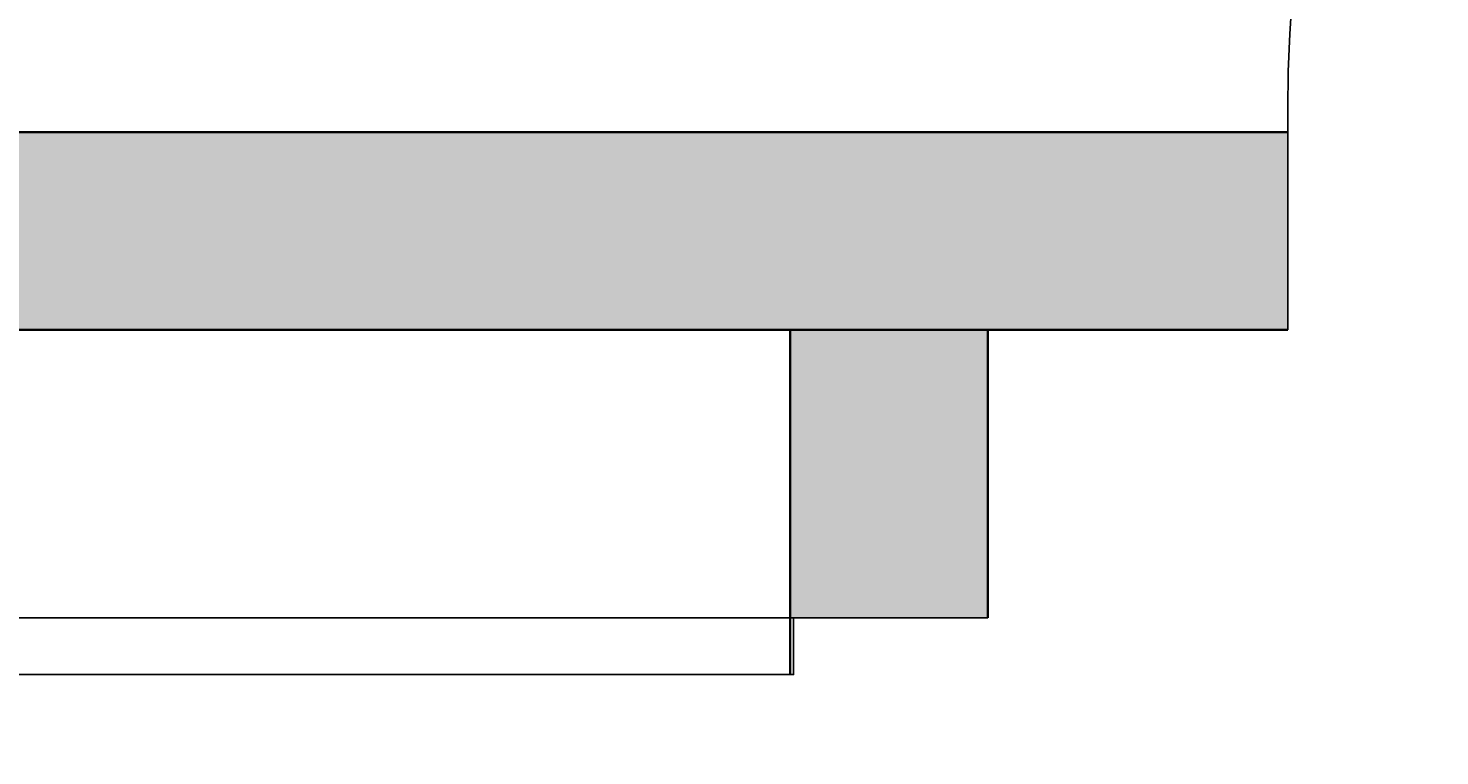
# Model space of a CAD drawing. Units: inches. Extents: x 1998 to 2588, y 1139 to 1977.
# Tile 66 of 134: x 2160 to 2192, y 1746 to 1762. Entities that reach past the tile are written whole.
import ezdxf

# ---------------------------------------------------------------- set-up
doc = ezdxf.new("R2010")
doc.units = ezdxf.units.IN
for name, color, linetype, lineweight in [('A-ANNO-DIMS', 2, 'Continuous', 18), ('A-WALL-PATT', 252, 'Continuous', 13), ('DOOR', 52, 'Continuous', 25), ('WALL', 200, 'Continuous', 35)]:
    doc.layers.add(name, color=color, linetype=linetype, lineweight=lineweight)
doc.styles.get("Standard").update_dxf_attribs({"font": 'arial.ttf'})
doc.dimstyles.get("Standard").update_dxf_attribs({"dimtxt": 0.18, "dimasz": 0.18, "dimexe": 0.18, "dimexo": 0.0625, "dimgap": 0.09, "dimtad": 0, "dimtih": 1, "dimtoh": 1, "dimdec": 4, "dimzin": 0, "dimdsep": 46, "dimtxsty": 'Standard', "dimcen": 0.09, "dimadec": 0, "dimazin": 0, "dimtfac": 1, "dimtdec": 4, "dimtofl": 0, "dimtmove": 0, "dimatfit": 3, "dimfxl": 1, "dimtolj": 1, "dimtzin": 0, "dimarcsym": 0})

# ---------------------------------------------------------------- blocks, each defined once
blk = doc.blocks.new('*U2')
for p, q in [((0, 0), (0, -6)), ((40, 0), (40, -6))]:
    blk.add_line(p, q)
blk.add_lwpolyline([(0, 0), (0, 40), (1.75, 40), (1.75, 0)], close=True)
blk.add_arc((0, 0), 40, 0, 90)
blk = doc.blocks.new('*D37')
at = {"layer": 'A-ANNO-DIMS', "color": 0, "lineweight": -2, "transparency": 16777216}
for p, q in [((2148.455, 1612.795), (2148.455, 1977.362)), ((2197.45, 1612.795), (2197.45, 1977.362)), ((2148.635, 1977.182), (2172.73, 1977.182)), ((2197.27, 1977.182), (2173.175, 1977.182))]:
    blk.add_line(p, q, dxfattribs=at)
at = {"layer": 'A-ANNO-DIMS', "color": 0, "transparency": 16777216}
for points in [[(2148.635, 1977.212), (2148.635, 1977.152), (2148.455, 1977.182)], [(2197.27, 1977.212), (2197.27, 1977.152), (2197.45, 1977.182)]]:
    blk.add_solid(points, dxfattribs=at)
at = {"layer": 'Defpoints', "color": 0, "transparency": 16777216}
for p in [(2197.45, 1977.182), (2148.455, 1612.732), (2197.45, 1612.732)]:
    blk.add_point(p, dxfattribs=at)
at = {"layer": 'A-ANNO-DIMS', "color": 0, "transparency": 16777216, "insert": (2172.952, 1977.182), "char_height": 0.18, "attachment_point": 5}
blk.add_mtext('\\A1;49', dxfattribs=at)

msp = doc.modelspace()

# ---------------------------------------------------------------- hatches: boundary and pattern name
at = {"layer": 'A-WALL-PATT'}
h = msp.add_hatch(color=256, dxfattribs=at)
h.dxf.hatch_style = 1
h.paths.add_polyline_path([(2222.9729, 1888.7324), (2099.4125, 1888.7324), (2099.4125, 1879.7324), (2222.9729, 1879.7324)])
h.paths.add_polyline_path([(2096.9729, 1868.3278), (2087.9729, 1868.3278), (2087.9729, 1775.637), (2096.9729, 1775.637)])
h.paths.add_polyline_path([(2227.4729, 1868.3278), (2222.9729, 1868.3278), (2222.9729, 1774.3318), (2227.4729, 1774.3318)])
h.paths.add_polyline_path([(2188.3019, 1759.7324), (2138.6074, 1759.7324), (2099.4125, 1759.7324), (2099.4125, 1755.2324), (2176.9729, 1755.2324), (2188.3019, 1755.2324)])
h.paths.add_polyline_path([(2087.9729, 1759.7324), (2059.4729, 1759.7324), (2059.4729, 1702.7324), (2087.9729, 1702.7324), (2087.9729, 1707.2324), (2063.9729, 1707.2324), (2063.9729, 1755.2324), (2087.9729, 1755.2324)])
h.paths.add_polyline_path([(2096.9729, 1755.2324), (2087.9729, 1755.2324), (2087.9729, 1707.2324), (2096.9729, 1707.2324)])
h.paths.add_polyline_path([(2187.0461, 1707.2324), (2105.9729, 1707.2324), (2096.9729, 1707.2324), (2087.9729, 1707.2324), (2087.9729, 1702.7324), (2105.9729, 1702.7324), (2114.9729, 1702.7324), (2187.0461, 1702.7324)])
h.paths.add_polyline_path([(2181.4729, 1719.2028), (2176.9729, 1719.2028), (2176.9729, 1707.2324), (2181.4729, 1707.2324)])
h.paths.add_polyline_path([(2216.0332, 1588.7324), (2114.9729, 1588.7324), (2105.9729, 1588.7324), (2105.9729, 1584.2324), (2216.0332, 1584.2324)])
h.paths.add_polyline_path([(2077.691, 1588.7324), (2061.4729, 1588.7324), (2061.4729, 1584.2324), (2077.691, 1584.2324)])
h.paths.add_polyline_path([(2105.9729, 1588.7324), (2098.0956, 1588.7324), (2098.0956, 1584.2324), (2105.9729, 1584.2324)])
h.paths.add_polyline_path([(2114.9729, 1596.2642), (2110.1012, 1596.2642), (2105.9729, 1596.2642), (2105.9729, 1588.7324), (2114.9729, 1588.7324)])
h.paths.add_polyline_path([(2114.9729, 1584.2324), (2105.9729, 1584.2324), (2105.9729, 1580.249), (2110.1012, 1580.249), (2114.9729, 1580.249)])
h.paths.add_polyline_path([(2114.9729, 1547.7716), (2110.1012, 1547.7716, -0.0318759), (2105.9729, 1548.035), (2105.9729, 1470.2324), (2108.3775, 1470.2324), (2108.3775, 1465.7324), (2186.2943, 1465.7324), (2186.2943, 1470.2324), (2114.9729, 1470.2324)])
h.paths.add_polyline_path([(2227.4729, 1584.2324), (2222.9729, 1584.2324), (2222.9729, 1486.137), (2227.4729, 1486.137)])
h.paths.add_polyline_path([(2295.4138, 1593.2324), (2227.4729, 1593.2324), (2227.4729, 1588.7324), (2295.4138, 1588.7324), (2295.4138, 1591.8729)])
h.paths.add_polyline_path([(2345.9729, 1627.1165), (2341.4729, 1627.1165), (2341.4729, 1593.2324), (2337.2869, 1593.2324), (2337.2869, 1591.8729), (2337.2869, 1588.7324), (2345.9729, 1588.7324)])
h.paths.add_polyline_path([(2291.9729, 1588.7324), (2287.4729, 1588.7324), (2287.4729, 1522.7324), (2291.9729, 1522.7324)])
h.paths.add_polyline_path([(2291.9729, 1522.7324), (2287.4729, 1522.7324), (2227.4729, 1522.7324), (2227.4729, 1518.2324), (2291.9729, 1518.2324)])
h.paths.add_polyline_path([(2295.7347, 1519.5919), (2295.7347, 1522.7324), (2291.9729, 1522.7324), (2291.9729, 1518.2324), (2295.7347, 1518.2324)])
h.paths.add_polyline_path([(2345.9729, 1522.7324), (2337.6078, 1522.7324), (2337.6078, 1519.5919), (2337.6078, 1518.2324), (2341.4729, 1518.2324), (2341.4729, 1488.5616), (2345.9729, 1488.5616)])
h.paths.add_polyline_path([(2345.9729, 1468.1569), (2341.4729, 1468.1569), (2341.4729, 1374.2324), (2227.4729, 1374.2324), (2227.4729, 1369.7324), (2345.9729, 1369.7324)])
h.paths.add_polyline_path([(2345.9729, 1369.7324), (2341.4729, 1369.7324), (2341.4729, 1362.2324), (2345.9729, 1362.2324)])
h.paths.add_polyline_path([(2345.9729, 1317.7324), (2345.9729, 1322.2324), (2341.4729, 1322.2324), (2341.4729, 1285.137), (2345.9729, 1285.137)], flags=17)
h.paths.add_polyline_path([(2356.2096, 1322.2324), (2345.9729, 1322.2324), (2345.9729, 1317.7324), (2356.2096, 1317.7324), (2356.2096, 1319.3088)], flags=17)
h.paths.add_polyline_path([(2393.9729, 1322.2324), (2375.6999, 1322.2324), (2375.6999, 1319.3088, -0.0202458), (2375.636, 1317.7324), (2393.9729, 1317.7324)], flags=17)
h.paths.add_polyline_path([(2398.4729, 1322.2324), (2393.9729, 1322.2324), (2393.9729, 1317.7324), (2393.9729, 1237.7324), (2345.9729, 1237.7324), (2345.9729, 1264.7324), (2341.4729, 1264.7324), (2341.4729, 1228.7324), (2393.9729, 1228.7324), (2482.7412, 1228.7324), (2482.7412, 1237.7324), (2398.4729, 1237.7324), (2398.4729, 1297.1029)])
h.paths.add_polyline_path([(2398.4729, 1362.2324), (2393.9729, 1362.2324), (2393.9729, 1357.7324), (2398.4729, 1357.7324)])
h.paths.add_polyline_path([(2345.9729, 1329.7549), (2341.4729, 1329.7549), (2341.4729, 1322.2324), (2345.9729, 1322.2324)])
h = msp.add_hatch(color=256, dxfattribs=at)
h.dxf.hatch_style = 1
h.paths.add_polyline_path([(2527.4729, 1362.2324), (2510.9729, 1362.2324), (2510.9729, 1357.7324), (2518.4729, 1357.7324), (2518.4729, 1237.7324), (2503.1458, 1237.7324), (2503.1458, 1228.7324), (2527.4729, 1228.7324)])
h.paths.add_polyline_path([(2490.5682, 1362.2324), (2398.4729, 1362.2324), (2398.4729, 1357.7324), (2490.5682, 1357.7324)])
h.paths.add_polyline_path([(2224.9729, 1264.7324), (2222.9729, 1264.7324), (2222.9729, 1232.4125), (2341.4729, 1232.4125), (2341.4729, 1234.4125), (2224.9729, 1234.4125)])
h.paths.add_polyline_path([(2334.5332, 1273.7324), (2264.7638, 1273.7324), (2264.7638, 1269.5611, -0.043659), (2264.3413, 1264.7324), (2334.5332, 1264.7324)])
h.paths.add_polyline_path([(2236.9551, 1273.7324), (2234.4125, 1273.7324), (2234.4125, 1264.7324), (2236.9551, 1264.7324), (2236.9551, 1269.5611)])
h.paths.add_polyline_path([(2222.9729, 1293.2324), (2096.9729, 1293.2324), (2096.9729, 1345.0966), (2087.9729, 1345.0966), (2087.9729, 1284.2324), (2222.9729, 1284.2324), (2222.9729, 1285.137)])
h.paths.add_polyline_path([(2096.9729, 1458.7927), (2087.9729, 1458.7927), (2087.9729, 1417.7324), (2087.9729, 1413.2324), (2096.9729, 1413.2324), (2096.9729, 1417.7324)])
h.paths.add_polyline_path([(2096.9729, 1413.2324), (2087.9729, 1413.2324), (2087.9729, 1365.5012), (2096.9729, 1365.5012), (2096.9729, 1369.3358)])
h.paths.add_polyline_path([(2186.2943, 1417.7324), (2138.6074, 1417.7324), (2096.9729, 1417.7324), (2096.9729, 1413.2324), (2138.6074, 1413.2324), (2186.2943, 1413.2324)])
h.paths.add_polyline_path([(2181.4729, 1465.7324), (2176.9729, 1465.7324), (2176.9729, 1451.6434), (2181.4729, 1451.6434)])
h.paths.add_polyline_path([(2181.4729, 1422.1664), (2176.9729, 1422.1664), (2176.9729, 1417.7324), (2181.4729, 1417.7324)])
h.paths.add_polyline_path([(2063.9729, 1465.7324), (2087.9729, 1465.7324), (2087.9729, 1470.2324), (2059.4729, 1470.2324), (2059.4729, 1413.2324), (2087.9729, 1413.2324), (2087.9729, 1417.7324), (2063.9729, 1417.7324)])
h.paths.add_polyline_path([(2181.4729, 1755.2324), (2176.9729, 1755.2324), (2176.9729, 1748.6798), (2177.0513, 1748.6798), (2181.4729, 1748.6798)])
h.paths.add_polyline_path([(2227.4729, 1707.2324), (2220.4647, 1707.2324), (2220.4647, 1702.7324), (2222.9729, 1702.7324), (2222.9729, 1604.637), (2227.4729, 1604.637)])
h.paths.add_polyline_path([(2114.9729, 1702.7324), (2105.9729, 1702.7324), (2105.9729, 1628.4781, -0.0318759), (2110.1012, 1628.7416), (2114.9729, 1628.7416)])
h.paths.add_polyline_path([(2345.9729, 1739.3278), (2341.4729, 1739.3278), (2341.4729, 1647.5211), (2345.9729, 1647.5211)])
h.paths.add_polyline_path([(2350.6273, 1641.2324), (2345.9729, 1641.2324), (2345.9729, 1636.7324), (2350.6273, 1636.7324), (2350.6273, 1639.8729)])
h.paths.add_polyline_path([(2501.9729, 1641.2324), (2407.9729, 1641.2324), (2392.5005, 1641.2324), (2392.5005, 1639.8729), (2392.5005, 1636.7324), (2501.9729, 1636.7324)])
h.paths.add_polyline_path([(2510.9729, 1755.2324), (2501.9729, 1755.2324), (2501.9729, 1641.2324), (2510.9729, 1641.2324)])
h.paths.add_polyline_path([(2549.1786, 1641.2324), (2522.3775, 1641.2324), (2522.3775, 1636.7324), (2540.1786, 1636.7324), (2540.1786, 1480.7324), (2522.3775, 1480.7324), (2522.3775, 1476.2324), (2549.1786, 1476.2324)])
h.paths.add_polyline_path([(2498.1786, 1594.7324), (2407.9729, 1594.7324), (2407.9729, 1585.7324), (2416.9729, 1585.7324), (2489.1786, 1585.7324), (2489.1786, 1531.7324), (2416.9729, 1531.7324), (2407.9729, 1531.7324), (2407.9729, 1522.7324), (2498.1786, 1522.7324)])
h.paths.add_polyline_path([(2351.6437, 1480.7324), (2345.9729, 1480.7324), (2345.9729, 1476.2324), (2351.6437, 1476.2324), (2351.6437, 1477.5919)])
h.paths.add_polyline_path([(2501.9729, 1480.7324), (2498.1786, 1480.7324), (2407.9729, 1480.7324), (2393.5168, 1480.7324), (2393.5168, 1477.5919), (2393.5168, 1476.2324), (2501.9729, 1476.2324)])

# ---------------------------------------------------------------- linework, layer by layer
at = {"layer": 'WALL'}
for p, q in [((2138.6074, 1759.7324), (2188.3019, 1759.7324)), ((2096.9729, 1755.2324), (2176.9729, 1755.2324)), ((2138.6074, 1755.2324), (2188.3019, 1755.2324)), ((2188.3019, 1755.2324), (2138.6074, 1755.2324)), ((2176.9729, 1755.2324), (2176.9729, 1747.3902)), ((2181.4729, 1755.2324), (2181.4729, 1748.6798))]:
    msp.add_line(p, q, dxfattribs=at)

# ---------------------------------------------------------------- block references
at = {"layer": 'DOOR', "xscale": -0.8354643497673233, "yscale": 0.8354643497673233, "zscale": 0.8354643497673233}
msp.add_blockref('*U2', (2221.7204, 1760.2452), dxfattribs=at)
at = {"layer": 'DOOR', "xscale": -0.736924595324625, "yscale": 0.736924595324625, "zscale": 0.736924595324625, "rotation": 90}
msp.add_blockref('*U2', (2177.0513, 1748.6798), dxfattribs=at)

# ---------------------------------------------------------------- dimensions: what is measured, and where the dimension line sits
at = {"layer": 'A-ANNO-DIMS'}
dim = msp.add_linear_dim(base=(2197.4499, 1977.1824), p1=(2148.4548, 1612.7324), p2=(2197.4499, 1612.7324), dimstyle='Standard', override={"dimdec": 0, "dimlfac": 1, "dimrnd": 0, "dimzin": 0, "dimdsep": 46, "dimlunit": 2}, dxfattribs=at)
dim.commit()
dim.dimension.update_dxf_attribs({"geometry": '*D37', "text_midpoint": (2172.9524, 1977.1824)})

doc.saveas('drawing.dxf')
